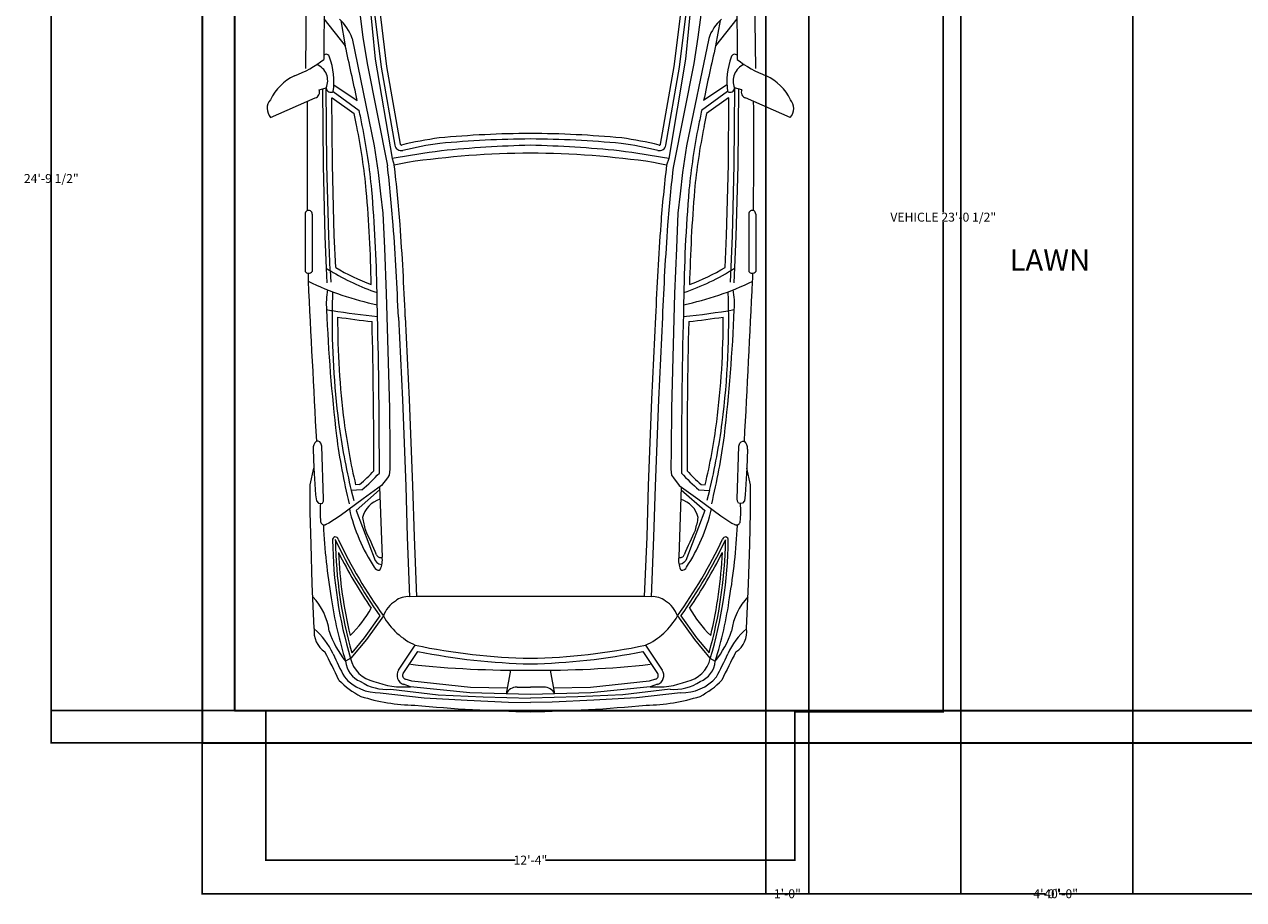
# Model space of a CAD drawing. Units: inches. Extents: x 594 to 1173, y 353 to 1285.
# Tile 1 of 6: x 594 to 934, y 355 to 600. Entities that reach past the tile are written whole.
import ezdxf

# ---------------------------------------------------------------- set-up
doc = ezdxf.new("R2010")
doc.units = ezdxf.units.IN
doc.header["$MEASUREMENT"] = 0
for name, color, linetype, lineweight in [('A-ANNO-DIMS', 2, 'Continuous', 18), ('A-AREA-IDEN', 7, 'Continuous', 25), ('C-PRKG-VEHI', 8, 'Continuous', 13), ('C-PROP', 7, 'Continuous', 35)]:
    doc.layers.add(name, color=color, linetype=linetype, lineweight=lineweight)
doc.styles.get("Standard").update_dxf_attribs({"font": 'arial.ttf'})
doc.dimstyles.get("Standard").update_dxf_attribs({"dimtxt": 2.5, "dimasz": 0.18, "dimexe": 0.18, "dimexo": 0.0625, "dimgap": 0.09, "dimtad": 0, "dimtih": 1, "dimtoh": 1, "dimzin": 0, "dimdsep": 46, "dimlunit": 3, "dimtxsty": 'Standard', "dimcen": 0.09, "dimadec": 0, "dimazin": 0, "dimtfac": 1, "dimtofl": 0, "dimtmove": 0, "dimatfit": 3, "dimfxl": 1, "dimtolj": 1, "dimtzin": 0, "dimarcsym": 0})

# ---------------------------------------------------------------- blocks, each defined once
blk = doc.blocks.new('A$C27D64469')
for p, q in [((-0.6398, -1.1535), (-0.5904, -1.5351)), ((-0.5908, -1.1535), (-0.5454, -1.6151)), ((0.618, -1.1535), (0.5726, -1.6151)), ((0.6669, -1.1535), (0.6175, -1.5351)), ((-0.563, -1.3311), (-0.5244, -1.6438)), ((-0.5431, -1.3287), (-0.5046, -1.6408)), ((0.5317, -1.6408), (0.5703, -1.3287)), ((0.5515, -1.6438), (0.5901, -1.3311)), ((-0.7946, -1.3764), (-0.7975, -1.6481)), ((-0.7302, -1.3933), (-0.7314, -1.6155)), ((0.7573, -1.3933), (0.7586, -1.6155)), ((0.8217, -1.3764), (0.8246, -1.6481)), ((-0.7306, -1.4695), (-0.6539, -1.5666)), ((-0.6702, -1.4746), (-0.6539, -1.5666)), ((0.7578, -1.4695), (0.681, -1.5666)), ((0.6973, -1.4746), (0.681, -1.5666)), ((-0.5904, -1.5351), (-0.5754, -1.6301)), ((0.6175, -1.5351), (0.6026, -1.6301)), ((-0.6294, -1.5396), (-0.5492, -1.9272)), ((0.6565, -1.5396), (0.5764, -1.9272)), ((-0.5454, -1.6151), (-0.4851, -1.9723)), ((0.5726, -1.6151), (0.5122, -1.9723)), ((-0.5754, -1.6301), (-0.5017, -1.9986)), ((-0.5244, -1.6438), (-0.475, -1.9247)), ((-0.5046, -1.6408), (-0.4553, -1.9213)), ((0.4824, -1.9213), (0.5317, -1.6408)), ((0.5021, -1.9247), (0.5515, -1.6438)), ((0.6026, -1.6301), (0.5289, -1.9986)), ((-0.6947, -1.7069), (-0.6109, -1.7637)), ((0.7218, -1.7069), (0.638, -1.7637)), ((-0.9228, -1.8245), (-0.7622, -1.7543)), ((-0.7483, -1.7248), (-0.7225, -1.7182)), ((-0.7364, -1.7217), (-0.7338, -1.998)), ((-0.7199, -1.9952), (-0.7225, -1.7182)), ((-0.6999, -1.9949), (-0.7021, -1.7537)), ((-0.7009, -1.7536), (-0.6216, -1.8108)), ((-0.6971, -1.7317), (-0.6035, -1.7992)), ((0.7242, -1.7317), (0.6307, -1.7992)), ((0.7281, -1.7536), (0.6487, -1.8108)), ((0.7271, -1.9949), (0.7293, -1.7537)), ((0.7496, -1.7182), (0.7471, -1.9952)), ((0.7755, -1.7248), (0.7496, -1.7182)), ((0.7635, -1.7217), (0.761, -1.998)), ((0.9499, -1.8245), (0.7893, -1.7543)), ((-0.5492, -1.9272), (-0.5351, -2.0233)), ((0.5764, -1.9272), (0.5623, -2.0233)), ((-0.4851, -1.9723), (-0.477, -1.9966)), ((0.5122, -1.9723), (0.5041, -1.9966)), ((-0.7338, -1.998), (-0.7273, -2.254)), ((-0.7134, -2.2512), (-0.7199, -1.9952)), ((-0.6934, -2.2505), (-0.6999, -1.9949)), ((0.7206, -2.2505), (0.7271, -1.9949)), ((0.7471, -1.9952), (0.7406, -2.2512)), ((0.761, -1.998), (0.7545, -2.254)), ((-0.5351, -2.0233), (-0.5266, -2.1005)), ((0.5623, -2.0233), (0.5538, -2.1005)), ((-0.5266, -2.1005), (-0.5182, -2.1702)), ((0.5538, -2.1005), (0.5453, -2.1702)), ((-0.7987, -2.1729), (-0.7987, -2.3802)), ((-0.7732, -2.1729), (-0.7732, -2.3802)), ((-0.5182, -2.1702), (-0.5125, -2.2965)), ((0.5453, -2.1702), (0.5397, -2.2965)), ((0.8003, -2.1729), (0.8003, -2.3802)), ((0.8259, -2.1729), (0.8259, -2.3802)), ((-0.7273, -2.254), (-0.7223, -2.368)), ((-0.7078, -2.3771), (-0.7134, -2.2512)), ((-0.6883, -2.3655), (-0.6934, -2.2505)), ((0.7155, -2.3655), (0.7206, -2.2505)), ((0.7406, -2.2512), (0.7332, -2.4181)), ((0.7545, -2.254), (0.7471, -2.4209)), ((-0.5125, -2.2965), (-0.5059, -2.4594)), ((0.5397, -2.2965), (0.5331, -2.4594)), ((-0.7223, -2.368), (-0.7199, -2.4209)), ((-0.7078, -2.3771), (-0.706, -2.4181)), ((-0.5059, -2.4594), (-0.4945, -2.8747)), ((0.5331, -2.4594), (0.5216, -2.8747)), ((-0.4622, -2.5454), (-0.4477, -2.8433)), ((-0.4375, -2.5434), (-0.423, -2.8413)), ((0.4646, -2.5434), (0.4501, -2.8413)), ((0.4894, -2.5454), (0.4748, -2.8433)), ((-0.4477, -2.8433), (-0.4357, -3.1539)), ((-0.423, -2.8413), (-0.4109, -3.152)), ((0.4501, -2.8413), (0.4381, -3.152)), ((0.4748, -2.8433), (0.4628, -3.1539)), ((-0.4945, -2.8747), (-0.4935, -3.0236)), ((0.5216, -2.8747), (0.5207, -3.0236)), ((-0.7694, -3.0205), (-0.7665, -3.0897)), ((-0.7516, -2.9924), (-0.758, -2.9914)), ((-0.7456, -2.9946), (-0.7516, -2.9924)), ((-0.7413, -2.9989), (-0.7456, -2.9946)), ((-0.738, -3.0096), (-0.7413, -2.9989)), ((-0.7319, -3.1994), (-0.738, -3.0096)), ((-0.4935, -3.0236), (-0.4926, -3.0933)), ((0.5207, -3.0236), (0.5197, -3.0933)), ((0.759, -3.1994), (0.7651, -3.0096)), ((0.7651, -3.0096), (0.7684, -2.9989)), ((0.7684, -2.9989), (0.7727, -2.9946)), ((0.7727, -2.9946), (0.7788, -2.9924)), ((0.7788, -2.9924), (0.7852, -2.9914)), ((0.7965, -3.0205), (0.7936, -3.0897)), ((-0.7802, -3.1498), (-0.7665, -3.0897)), ((-0.7665, -3.0897), (-0.761, -3.1849)), ((-0.4954, -3.115), (-0.502, -3.1244)), ((-0.4926, -3.0933), (-0.4954, -3.115)), ((0.5197, -3.0933), (0.5226, -3.115)), ((0.5226, -3.115), (0.5292, -3.1244)), ((0.7936, -3.0897), (0.7882, -3.1849)), ((0.8074, -3.1498), (0.7936, -3.0897)), ((-0.7802, -3.248), (-0.7802, -3.1498)), ((-0.6019, -3.1478), (-0.6165, -3.1489)), ((-0.5227, -3.1517), (-0.5896, -3.1998)), ((-0.5302, -3.1571), (-0.5208, -3.4098)), ((-0.502, -3.1244), (-0.5227, -3.1517)), ((-0.4357, -3.1539), (-0.4303, -3.3385)), ((-0.4109, -3.152), (-0.4055, -3.3366)), ((0.4381, -3.152), (0.4327, -3.3366)), ((0.4628, -3.1539), (0.4574, -3.3385)), ((0.5292, -3.1244), (0.5499, -3.1517)), ((0.5573, -3.1571), (0.548, -3.4098)), ((0.5499, -3.1517), (0.6167, -3.1998)), ((0.6291, -3.1478), (0.6437, -3.1489)), ((0.8074, -3.248), (0.8074, -3.1498)), ((-0.761, -3.1849), (-0.7577, -3.207)), ((-0.7577, -3.207), (-0.7506, -3.2153)), ((-0.7324, -3.2087), (-0.7319, -3.1994)), ((-0.5896, -3.1998), (-0.6725, -3.261)), ((-0.594, -3.1673), (-0.632, -3.1701)), ((-0.632, -3.1701), (-0.6229, -3.206)), ((-0.5298, -3.1676), (-0.615, -3.2421)), ((0.557, -3.1676), (0.6422, -3.2421)), ((0.6167, -3.1998), (0.6996, -3.261)), ((0.6212, -3.1673), (0.6592, -3.1701)), ((0.6592, -3.1701), (0.65, -3.206)), ((0.7595, -3.2087), (0.759, -3.1994)), ((0.7849, -3.207), (0.7778, -3.2153)), ((0.7882, -3.1849), (0.7849, -3.207)), ((-0.777, -3.3641), (-0.7802, -3.248)), ((-0.7506, -3.2153), (-0.743, -3.2171)), ((-0.743, -3.2171), (-0.7359, -3.2158)), ((-0.7359, -3.2158), (-0.7324, -3.2087)), ((-0.615, -3.2421), (-0.5463, -3.4221)), ((0.6422, -3.2421), (0.5734, -3.4221)), ((0.7631, -3.2158), (0.7595, -3.2087)), ((0.7702, -3.2171), (0.7631, -3.2158)), ((0.7778, -3.2153), (0.7702, -3.2171)), ((0.8042, -3.3641), (0.8074, -3.248)), ((-0.7224, -3.2921), (-0.7327, -3.2955)), ((-0.713, -3.2874), (-0.7233, -3.2925)), ((-0.6725, -3.261), (-0.713, -3.2874)), ((0.6996, -3.261), (0.7401, -3.2874)), ((0.7401, -3.2874), (0.7505, -3.2925)), ((0.7495, -3.2921), (0.7599, -3.2955)), ((-0.4303, -3.3385), (-0.4218, -3.5529)), ((-0.4055, -3.3366), (-0.3971, -3.5519)), ((0.4327, -3.3366), (0.4242, -3.5519)), ((0.4574, -3.3385), (0.449, -3.5529)), ((-0.7728, -3.5066), (-0.777, -3.3641)), ((0.8, -3.5066), (0.8042, -3.3641)), ((-0.5463, -3.4221), (-0.5397, -3.4296)), ((0.5734, -3.4221), (0.5668, -3.4296)), ((-0.5397, -3.4296), (-0.5331, -3.4343)), ((-0.5331, -3.4343), (-0.5217, -3.4366)), ((0.5602, -3.4343), (0.5488, -3.4366)), ((0.5668, -3.4296), (0.5602, -3.4343)), ((-0.7654, -3.667), (-0.7728, -3.5066)), ((0.7926, -3.667), (0.8, -3.5066)), ((-0.3971, -3.5519), (-0.4218, -3.5529)), ((0.0136, -3.5519), (-0.3971, -3.5519)), ((0.4242, -3.5519), (0.0136, -3.5519)), ((0.449, -3.5529), (0.4242, -3.5519)), ((-0.5287, -3.6221), (-0.5854, -3.701)), ((-0.5163, -3.6221), (-0.5774, -3.7071)), ((0.5435, -3.6221), (0.6046, -3.7071)), ((0.5559, -3.6221), (0.6126, -3.701)), ((-0.5774, -3.7071), (-0.6331, -3.7742)), ((-0.5854, -3.701), (-0.6302, -3.755)), ((-0.4616, -3.818), (-0.4014, -3.7275)), ((0.4285, -3.7275), (0.4887, -3.818)), ((0.6046, -3.7071), (0.6602, -3.7742)), ((0.6126, -3.701), (0.6574, -3.755)), ((-0.6331, -3.7742), (-0.6525, -3.7849)), ((-0.4449, -3.8291), (-0.3922, -3.7498)), ((0.4193, -3.7498), (0.4721, -3.8291)), ((0.6602, -3.7742), (0.6796, -3.7849)), ((-0.0581, -3.8176), (-0.0735, -3.9028)), ((0.0853, -3.8176), (0.1006, -3.9028)), ((-0.4142, -3.8575), (-0.4379, -3.8496)), ((-0.2029, -3.8795), (-0.4142, -3.8575)), ((0.4414, -3.8575), (0.2301, -3.8795)), ((0.465, -3.8496), (0.4414, -3.8575)), ((-0.5278, -3.8988), (-0.3693, -3.9174)), ((-0.4897, -3.8861), (-0.3195, -3.9066)), ((-0.4185, -3.8772), (-0.4442, -3.8686)), ((-0.2042, -3.8994), (-0.4185, -3.8772)), ((-0.3195, -3.9066), (-0.1571, -3.9135)), ((0.0136, -3.905), (-0.2042, -3.8994)), ((-0.0699, -3.8829), (-0.2029, -3.8795)), ((-0.0347, -3.8792), (0.0136, -3.8792)), ((0.0618, -3.8792), (0.0136, -3.8792)), ((0.2314, -3.8994), (0.0136, -3.905)), ((0.2301, -3.8795), (0.097, -3.8829)), ((0.3466, -3.9066), (0.1842, -3.9135)), ((0.4456, -3.8772), (0.2314, -3.8994)), ((0.5168, -3.8861), (0.3466, -3.9066)), ((0.5549, -3.8988), (0.3965, -3.9174)), ((0.4713, -3.8686), (0.4456, -3.8772)), ((-0.3693, -3.9174), (-0.2148, -3.9262)), ((-0.2148, -3.9262), (-0.0652, -3.933)), ((-0.1571, -3.9135), (0.0136, -3.9184)), ((-0.0652, -3.933), (0.0136, -3.934)), ((0.1842, -3.9135), (0.0136, -3.9184)), ((0.0923, -3.933), (0.0136, -3.934)), ((0.242, -3.9262), (0.0923, -3.933)), ((0.3965, -3.9174), (0.242, -3.9262))]:
    blk.add_line(p, q)
for centre, radius, start, end in [((-0.7826, -1.5905), 0.1615, 18.3646, 48.2784), ((0.8098, -1.5905), 0.1615, 131.7216, 161.6354), ((-10.825, -3.8887), 10.4328, 11.75206, 12.86028), ((10.8521, -3.8887), 10.4328, 167.13972, 168.24794), ((-0.9818, -1.2945), 0.4071, 290.8732, 307.9458), ((-0.7227, -1.6094), 0.0124, 11.3416, 134.5987), ((-0.9441, -1.6953), 0.2497, 351.6082, 20.7105), ((0.9712, -1.6953), 0.2497, 159.2895, 188.3918), ((0.7498, -1.6094), 0.0124, 45.4013, 168.6584), ((1.0089, -1.2945), 0.4071, 232.0542, 249.1268), ((-0.7801, -1.6924), 0.0631, 335.8522, 68.2516), ((0.8072, -1.6924), 0.0631, 111.7484, 204.1478), ((-0.7607, -1.8385), 0.1804, 114.9135, 154.5523), ((0.7879, -1.8385), 0.1804, 25.4477, 65.0865), ((-0.7685, -1.7333), 0.0219, 286.784, 22.9417), ((-0.7054, -1.7168), 0.0171, 184.6651, 299.1967), ((-0.7054, -1.7168), 0.0371, 275.0842, 276.9824), ((0.7326, -1.7168), 0.0171, 240.8033, 355.3349), ((0.7326, -1.7168), 0.0371, 263.0176, 264.9158), ((0.7957, -1.7333), 0.0219, 157.0583, 253.216), ((-0.8877, -1.7923), 0.0477, 138.9599, 222.5475), ((28.5723, -1.9291), 29.3639, 179.68363, 180.45247), ((-10.825, -3.8887), 10.4328, 11.24656, 11.5533), ((10.8521, -3.8887), 10.4328, 168.4467, 168.75344), ((-28.5452, -1.9291), 29.3639, 359.54753, 0.31637), ((0.9148, -1.7923), 0.0477, 317.4525, 41.0401), ((-10.825, -3.8887), 10.4128, 11.24635, 11.51036), ((10.8521, -3.8887), 10.4128, 168.48964, 168.75365), ((-2.7812, -2.2979), 2.2132, 5.4405, 11.4681), ((-2.7812, -2.2979), 2.2332, 5.4374, 11.4671), ((0.034, -5.6085), 3.7262, 90.3146, 95.3817), ((-0.0069, -5.6085), 3.7262, 84.6183, 89.6854), ((2.8083, -2.2979), 2.2332, 168.5329, 174.5626), ((2.8083, -2.2979), 2.2132, 168.5319, 174.5595), ((-0.4518, -1.9207), 0.0236, 189.9743, 283.4471), ((-0.4518, -1.9207), 0.00357, 189.9743, 283.4471), ((-0.1284, -3.2729), 1.3868, 97.7498, 103.4471), ((-0.1284, -3.2729), 1.3668, 97.7671, 103.4471), ((0.034, -5.6085), 3.7062, 90.3163, 95.3753), ((0.1214, -6.2334), 4.3098, 91.434, 95.7038), ((-0.0069, -5.6085), 3.7062, 84.6247, 89.6837), ((-0.0943, -6.2334), 4.3098, 84.2962, 88.566), ((0.1556, -3.2729), 1.3668, 76.5529, 82.2329), ((0.1556, -3.2729), 1.3868, 76.5529, 82.2502), ((0.4789, -1.9207), 0.0236, 256.5529, 350.0257), ((0.4789, -1.9207), 0.00357, 256.5529, 350.0257), ((2.8455, -23.0231), 21.3127, 98.50598, 98.99062), ((0.0355, -5.2091), 3.2558, 90.3851, 98.2136), ((-0.0083, -5.2091), 3.2558, 81.7864, 89.6149), ((-2.8184, -23.0231), 21.3127, 81.00938, 81.49402), ((-6.4408, -2.6841), 5.9785, 4.51893, 6.58421), ((-0.0958, -3.6836), 1.7295, 101.1311, 102.7329), ((-6.416, -2.6821), 5.9785, 4.51893, 6.58421), ((0.1229, -3.6836), 1.7295, 77.2671, 78.8689), ((6.4432, -2.6821), 5.9785, 173.41579, 175.48107), ((6.4679, -2.6841), 5.9785, 173.41579, 175.48107), ((-6.2705, -2.56), 5.7121, 1.3286, 4.7387), ((-6.2705, -2.56), 5.7321, 1.03863, 4.73991), ((6.2976, -2.56), 5.7321, 175.26009, 179.33379), ((6.2976, -2.56), 5.7121, 175.2613, 178.6714), ((-0.7859, -2.1729), 0.0128, 359.8097, 180.1903), ((0.8131, -2.1729), 0.0128, 359.8097, 180.1903), ((-11.1621, -2.9794), 10.7086, 2.32274, 4.10377), ((-11.1373, -2.9775), 10.7086, 2.32274, 4.10377), ((11.1645, -2.9775), 10.7086, 175.89623, 177.67726), ((11.1892, -2.9794), 10.7086, 175.89623, 177.67726), ((-0.2816, -1.6867), 0.8114, 237.1024, 238.3082), ((-0.2816, -1.6867), 0.7914, 239.0709, 249.4088), ((0.3087, -1.6867), 0.8114, 288.5207, 302.8976), ((0.3087, -1.6867), 0.7914, 290.5912, 300.9291), ((-0.7859, -2.3704), 0.0161, 217.6419, 322.3581), ((28.5723, -1.9291), 29.3639, 180.89229, 180.9487), ((145.5619, 4.7984), 146.5271, 182.82189, 183.047472), ((-0.3074, -1.4152), 1.1094, 244.3519, 257.9711), ((-0.2816, -1.6867), 0.8114, 238.3082, 251.4793), ((0.3345, -1.4152), 1.1094, 282.0289, 295.6481), ((-145.5348, 4.7984), 146.5271, 356.952528, 357.17811), ((0.8131, -2.3704), 0.0161, 217.6419, 322.3581), ((-28.5452, -1.9291), 29.3639, 359.0513, 359.10771), ((-0.4463, -2.4963), 0.2758, 169.4971, 184.519), ((2.1845, -2.5566), 2.8858, 177.9428, 179.2929), ((-6.2705, -2.56), 5.7321, 0.66621, 1.03863), ((-2.1573, -2.5566), 2.8858, 352.6735, 2.0572), ((0.4735, -2.4963), 0.2758, 355.481, 10.5029), ((-21.144, -3.0635), 20.6131, 1.44842, 1.58522), ((21.1711, -3.0635), 20.6131, 178.41478, 180.12035), ((-0.2547, 0.2402), 2.7971, 260.3968, 260.8181), ((5.4584, -2.2589), 6.1852, 182.40058, 186.62429), ((2.1845, -2.5566), 2.8858, 179.2929, 187.3265), ((-0.2547, 0.2402), 2.7971, 260.8181, 264.1988), ((-0.2547, 0.2402), 2.8171, 261.2916, 263.8402), ((2.1845, -2.5566), 2.8658, 179.7551, 187.3262), ((-21.144, -3.0635), 20.6131, 359.87965, 1.44842), ((0.2819, 0.2402), 2.7971, 275.8012, 279.6032), ((0.2819, 0.2402), 2.8171, 276.1598, 278.7084), ((-2.1573, -2.5566), 2.8658, 352.6738, 0.2449), ((-5.4313, -2.2589), 6.1852, 353.37571, 357.59942), ((-21.144, -3.0635), 20.5931, 359.90118, 1.39956), ((21.1711, -3.0635), 20.5931, 178.60044, 180.09882), ((1.5917, -2.6291), 2.2886, 187.4191, 193.6744), ((1.5917, -2.6291), 2.2686, 187.4195, 193.2465), ((-1.5646, -2.6291), 2.2686, 346.7535, 352.5805), ((-1.5646, -2.6291), 2.2886, 346.3256, 352.5809), ((1.584, -2.6769), 2.2886, 187.4191, 193.6744), ((-1.5568, -2.6769), 2.2886, 346.3256, 352.5809), ((-0.7323, -3.0182), 0.0371, 133.8458, 183.4773), ((0.7594, -3.0182), 0.0371, 356.5227, 46.1542), ((-0.9762, -2.7051), 0.5797, 310.2112, 317.1922), ((-0.9762, -2.7051), 0.5997, 309.5861, 317.9444), ((1.0033, -2.7051), 0.5997, 222.0556, 230.4139), ((1.0033, -2.7051), 0.5797, 222.8078, 229.7888), ((-0.5023, -3.2896), 0.0919, 106.6274, 166.1462), ((0.5294, -3.2896), 0.0919, 13.8538, 73.3726), ((-0.4258, -3.2462), 0.3189, 174.7532, 186.4501), ((-0.0025, -3.0882), 0.6536, 193.0984, 213.2489), ((0.0296, -3.0882), 0.6536, 326.7511, 346.9016), ((0.4529, -3.2462), 0.3189, 353.5499, 5.2468), ((-0.7293, -3.2805), 0.0135, 186.4501, 296.5725), ((1.5487, -3.1796), 2.2844, 182.9075, 189.515), ((-0.2573, -3.2127), 0.3386, 189.3185, 197.018), ((0.2844, -3.2127), 0.3386, 342.982, 350.6815), ((-1.5216, -3.1796), 2.2844, 350.485, 357.0925), ((0.7565, -3.2805), 0.0135, 243.4275, 353.5499), ((-0.6895, -3.3475), 0.0103, 9.7306, 189.7306), ((-6.7047, -6.1366), 6.7437, 23.9284, 24.763), ((6.7318, -6.1366), 6.7437, 155.237, 156.0716), ((0.7166, -3.3475), 0.0103, 350.2694, 170.2694), ((0.8768, -3.3275), 1.5766, 180.7904, 196.499), ((-0.6895, -3.3475), 0.000207, 234.3096, 189.7306), ((-0.6997, -3.3492), 0.0101, 0.7904, 9.7306), ((0.9825, -2.5519), 1.8518, 205.4494, 215.3046), ((0.8768, -3.3275), 1.5665, 180.7904, 195.8378), ((0.9825, -2.5519), 1.8417, 205.5332, 215.5287), ((-0.9554, -2.5519), 1.8417, 324.4713, 334.4668), ((-0.9554, -2.5519), 1.8518, 324.6954, 334.5506), ((-0.8496, -3.3275), 1.5665, 344.1622, 359.2096), ((-0.8496, -3.3275), 1.5766, 343.501, 359.2096), ((0.7166, -3.3475), 0.000207, 350.2694, 305.6904), ((0.7268, -3.3492), 0.0101, 170.2694, 179.2096), ((0.8768, -3.3275), 1.5564, 182.4426, 193.5531), ((0.9825, -2.5519), 1.8619, 206.8832, 214.0379), ((-0.5273, -3.3975), 0.0139, 196.0998, 297.49), ((-0.5991, -3.4208), 0.079, 335.0797, 7.9846), ((0.6263, -3.4208), 0.079, 172.0154, 204.9203), ((0.5544, -3.3975), 0.0139, 242.51, 343.9002), ((-0.9554, -2.5519), 1.8619, 325.9621, 333.1168), ((-0.8496, -3.3275), 1.5564, 346.4469, 357.5574), ((-0.5332, -3.4402), 0.0172, 201.6995, 279.6425), ((-0.5326, -3.4521), 0.00559, 294.9923, 338.6694), ((0.5598, -3.4521), 0.00559, 201.3306, 245.0077), ((0.5603, -3.4402), 0.0172, 260.3575, 338.3005), ((-0.931, -3.7054), 0.2213, 7.498, 43.5729), ((0.6722, -3.364), 1.3899, 187.9913, 197.6257), ((-0.4293, -3.6198), 0.0673, 83.5915, 130.4352), ((0.4565, -3.6198), 0.0673, 49.5648, 96.4085), ((-0.645, -3.364), 1.3899, 342.3743, 352.0087), ((0.9581, -3.7054), 0.2213, 136.4271, 172.502), ((-0.9014, -3.4088), 0.388, 313.0938, 331.4872), ((-0.421, -3.6549), 0.1008, 121.0416, 161.032), ((0.4482, -3.6549), 0.1008, 18.968, 58.9584), ((0.9285, -3.4088), 0.388, 208.5128, 226.9062), ((-0.3005, -3.502), 0.247, 209.0915, 245.8956), ((0.3276, -3.502), 0.247, 294.1044, 330.9085), ((-0.6785, -3.679), 0.0877, 172.132, 236.2396), ((-0.9429, -3.8711), 0.2695, 24.6265, 48.8595), ((-0.3962, -3.5747), 0.3315, 197.8909, 219.3552), ((0.4233, -3.5747), 0.3315, 320.6448, 342.1091), ((0.97, -3.8711), 0.2695, 131.1405, 155.3735), ((0.7057, -3.679), 0.0877, 303.7604, 7.868), ((0.0567, -1.5526), 2.2226, 258.1061, 268.8881), ((-0.0296, -1.5526), 2.2226, 271.1119, 281.8939), ((-3.375, -5.1387), 2.9889, 25.4724, 27.6425), ((0.5567, -3.1915), 1.3769, 204.3314, 208.2014), ((-0.528, -3.7506), 0.1097, 192.9436, 258.3207), ((0.0567, -1.5526), 2.2426, 258.453, 268.898), ((-0.0296, -1.5526), 2.2426, 271.102, 281.547), ((0.5551, -3.7506), 0.1097, 281.6793, 347.0564), ((-0.5295, -3.1915), 1.3769, 331.7986, 335.6686), ((3.4021, -5.1387), 2.9889, 152.3575, 154.5276), ((-0.566, -3.7782), 0.0867, 184.4324, 248.21), ((-0.4335, -3.8367), 0.0337, 146.3764, 251.5583), ((-0.0346, -0.3333), 3.4843, 263.6749, 270.7924), ((0.0618, -0.3333), 3.4843, 269.2076, 276.3251), ((0.4607, -3.8367), 0.0337, 288.4417, 33.6236), ((0.5932, -3.7782), 0.0867, 291.79, 355.5676), ((-0.4633, -3.6496), 0.2949, 223.6549, 242.8613), ((-0.5341, -3.738), 0.1609, 220.3568, 272.2613), ((-0.5047, -3.7168), 0.17, 236.6049, 275.0704), ((-0.4436, -3.5867), 0.2916, 248.5479, 274.9353), ((-0.4335, -3.8367), 0.0137, 146.3764, 251.5583), ((0.4707, -3.5867), 0.2916, 265.0647, 291.4521), ((0.4607, -3.8367), 0.0137, 288.4417, 33.6236), ((0.5318, -3.7168), 0.17, 264.9296, 303.3951), ((0.5613, -3.738), 0.1609, 267.7387, 319.6432), ((0.4904, -3.6496), 0.2949, 297.1387, 316.3451), ((-0.0379, -3.9176), 0.0386, 85.1824, 157.357), ((0.065, -3.9176), 0.0386, 22.643, 94.8176), ((-0.3932, -3.2709), 0.673, 252.2974, 269.1096), ((0.1171, 1.5736), 5.542, 264.6089, 268.93), ((-0.0899, 1.5736), 5.542, 271.07, 275.3911), ((0.4203, -3.2709), 0.673, 270.8904, 287.7026)]:
    blk.add_arc(centre, radius, start, end)
blk = doc.blocks.new('*D44')
at = {"layer": 'A-ANNO-DIMS', "color": 0, "lineweight": -2, "transparency": 16777216}
for p, q in [((808.99, 683.97), (850.58, 683.97)), ((850.4, 683.79), (850.4, 547.1)), ((850.4, 407.65), (850.4, 544.34)), ((808.99, 407.47), (850.58, 407.47))]:
    blk.add_line(p, q, dxfattribs=at)
at = {"layer": 'A-ANNO-DIMS', "color": 0, "transparency": 16777216}
for points in [[(850.37, 683.79), (850.43, 683.79), (850.4, 683.97)], [(850.37, 407.65), (850.43, 407.65), (850.4, 407.47)]]:
    blk.add_solid(points, dxfattribs=at)
at = {"layer": 'Defpoints', "color": 0, "transparency": 16777216}
for p in [(808.93, 683.97), (850.4, 683.97), (808.93, 407.47)]:
    blk.add_point(p, dxfattribs=at)
at = {"layer": 'A-ANNO-DIMS', "color": 0, "transparency": 16777216, "insert": (850.4, 545.72), "char_height": 2.5, "attachment_point": 5}
blk.add_mtext('\\A1;VEHICLE 23\'-0 1/2"', dxfattribs=at)
blk = doc.blocks.new('*D45')
at = {"layer": 'A-ANNO-DIMS', "color": 0, "lineweight": -2, "transparency": 16777216}
for p, q in [((661.13, 407.41), (661.13, 365.81)), ((808.93, 407.41), (808.93, 365.81)), ((661.31, 365.99), (730.76, 365.99)), ((808.75, 365.99), (739.29, 365.99))]:
    blk.add_line(p, q, dxfattribs=at)
at = {"layer": 'A-ANNO-DIMS', "color": 0, "transparency": 16777216}
for points in [[(661.31, 366.02), (661.31, 365.96), (661.13, 365.99)], [(808.75, 366.02), (808.75, 365.96), (808.93, 365.99)]]:
    blk.add_solid(points, dxfattribs=at)
at = {"layer": 'Defpoints', "color": 0, "transparency": 16777216}
for p in [(661.13, 407.47), (808.93, 407.47), (808.93, 365.99)]:
    blk.add_point(p, dxfattribs=at)
at = {"layer": 'A-ANNO-DIMS', "color": 0, "transparency": 16777216, "insert": (735.03, 365.99), "char_height": 2.5, "attachment_point": 5}
blk.add_mtext('\\A1;12\'-4"', dxfattribs=at)
blk = doc.blocks.new('*D46')
at = {"layer": 'A-ANNO-DIMS', "color": 0, "lineweight": -2, "transparency": 16777216}
for p, q in [((643.34, 398.72), (643.34, 356.4)), ((1123.34, 398.72), (1123.34, 356.4)), ((643.52, 356.58), (878.9, 356.58)), ((1123.16, 356.58), (887.77, 356.58))]:
    blk.add_line(p, q, dxfattribs=at)
at = {"layer": 'A-ANNO-DIMS', "color": 0, "transparency": 16777216}
for points in [[(643.52, 356.61), (643.52, 356.55), (643.34, 356.58)], [(1123.16, 356.61), (1123.16, 356.55), (1123.34, 356.58)]]:
    blk.add_solid(points, dxfattribs=at)
at = {"layer": 'Defpoints', "color": 0, "transparency": 16777216}
for p in [(643.34, 398.78), (1123.34, 398.78), (1123.34, 356.58)]:
    blk.add_point(p, dxfattribs=at)
at = {"layer": 'A-ANNO-DIMS', "color": 0, "transparency": 16777216, "insert": (883.34, 356.58), "char_height": 2.5, "attachment_point": 5}
blk.add_mtext('\\A1;40\'-0"', dxfattribs=at)
blk = doc.blocks.new('*D47')
at = {"layer": 'A-ANNO-DIMS', "color": 0, "lineweight": -2, "transparency": 16777216}
for p, q in [((643.27, 1238.78), (600.96, 1238.78)), ((601.14, 1238.6), (601.14, 820.15)), ((601.14, 398.96), (601.14, 817.42)), ((643.27, 398.78), (600.96, 398.78))]:
    blk.add_line(p, q, dxfattribs=at)
at = {"layer": 'A-ANNO-DIMS', "color": 0, "transparency": 16777216}
for points in [[(601.11, 1238.6), (601.17, 1238.6), (601.14, 1238.78)], [(601.11, 398.96), (601.17, 398.96), (601.14, 398.78)]]:
    blk.add_solid(points, dxfattribs=at)
at = {"layer": 'Defpoints', "color": 0, "transparency": 16777216}
for p in [(601.14, 1238.78), (643.34, 1238.78), (643.34, 398.78)]:
    blk.add_point(p, dxfattribs=at)
at = {"layer": 'A-ANNO-DIMS', "color": 0, "transparency": 16777216, "insert": (601.14, 818.78), "char_height": 2.5, "attachment_point": 5}
blk.add_mtext('\\A1;70\'-0"', dxfattribs=at)
blk = doc.blocks.new('*D56')
at = {"layer": 'A-ANNO-DIMS', "color": 0, "lineweight": -2, "transparency": 16777216}
for p, q in [((652.27, 705.28), (600.96, 705.28)), ((601.14, 705.1), (601.14, 557.92)), ((601.14, 407.96), (601.14, 555.15)), ((652.27, 407.78), (600.96, 407.78))]:
    blk.add_line(p, q, dxfattribs=at)
at = {"layer": 'A-ANNO-DIMS', "color": 0, "transparency": 16777216}
for points in [[(601.11, 705.1), (601.17, 705.1), (601.14, 705.28)], [(601.11, 407.96), (601.17, 407.96), (601.14, 407.78)]]:
    blk.add_solid(points, dxfattribs=at)
at = {"layer": 'Defpoints', "color": 0, "transparency": 16777216}
for p in [(601.14, 705.28), (652.34, 705.28), (652.34, 407.78)]:
    blk.add_point(p, dxfattribs=at)
at = {"layer": 'A-ANNO-DIMS', "color": 0, "transparency": 16777216, "insert": (601.14, 556.53), "char_height": 2.5, "attachment_point": 5}
blk.add_mtext('\\A1;24\'-9 1/2"', dxfattribs=at)
blk = doc.blocks.new('*D69')
at = {"layer": 'A-ANNO-DIMS', "color": 0, "lineweight": -2, "transparency": 16777216}
for p, q in [((855.34, 726.2), (855.34, 356.4)), ((903.34, 726.2), (903.34, 356.4)), ((855.52, 356.58), (875.87, 356.58)), ((903.16, 356.58), (882.8, 356.58))]:
    blk.add_line(p, q, dxfattribs=at)
at = {"layer": 'A-ANNO-DIMS', "color": 0, "transparency": 16777216}
for points in [[(855.52, 356.61), (855.52, 356.55), (855.34, 356.58)], [(903.16, 356.61), (903.16, 356.55), (903.34, 356.58)]]:
    blk.add_solid(points, dxfattribs=at)
at = {"layer": 'Defpoints', "color": 0, "transparency": 16777216}
for p in [(855.34, 726.26), (903.34, 726.26), (903.34, 356.58)]:
    blk.add_point(p, dxfattribs=at)
at = {"layer": 'A-ANNO-DIMS', "color": 0, "transparency": 16777216, "insert": (879.34, 356.58), "char_height": 2.5, "attachment_point": 5}
blk.add_mtext('\\A1;4\'-0"', dxfattribs=at)
blk = doc.blocks.new('*D73')
at = {"layer": 'A-ANNO-DIMS', "color": 0, "lineweight": -2, "transparency": 16777216}
for p, q in [((800.84, 870.22), (800.84, 356.4)), ((812.84, 870.22), (812.84, 356.4)), ((801.02, 356.58), (803.54, 356.58)), ((812.66, 356.58), (810.13, 356.58))]:
    blk.add_line(p, q, dxfattribs=at)
at = {"layer": 'A-ANNO-DIMS', "color": 0, "transparency": 16777216}
for points in [[(801.02, 356.61), (801.02, 356.55), (800.84, 356.58)], [(812.66, 356.61), (812.66, 356.55), (812.84, 356.58)]]:
    blk.add_solid(points, dxfattribs=at)
at = {"layer": 'Defpoints', "color": 0, "transparency": 16777216}
for p in [(800.84, 870.28), (812.84, 870.28), (812.84, 356.58)]:
    blk.add_point(p, dxfattribs=at)
at = {"layer": 'A-ANNO-DIMS', "color": 0, "transparency": 16777216, "insert": (806.84, 356.58), "char_height": 2.5, "attachment_point": 5}
blk.add_mtext('\\A1;1\'-0"', dxfattribs=at)

msp = doc.modelspace()

# ---------------------------------------------------------------- linework, layer by layer
at = {"layer": 'C-PROP'}
for p, q in [((643.337, 1238.783), (643.337, 398.783)), ((652.337, 1229.783), (652.337, 407.783)), ((652.337, 407.783), (1114.337, 407.783)), ((643.337, 398.783), (1123.337, 398.783))]:
    msp.add_line(p, q, dxfattribs=at)

# ---------------------------------------------------------------- block references
at = {"layer": 'C-PRKG-VEHI', "xscale": 77.53069963048091, "yscale": 77.53069963048091, "zscale": 77.53069963048091}
msp.add_blockref('A$C27D64469', (733.975, 715.065), dxfattribs=at)

# ---------------------------------------------------------------- texts
at = {"layer": 'A-AREA-IDEN'}
msp.add_text('LAWN', height=6, dxfattribs=at).set_placement((868.928, 530.726))

# ---------------------------------------------------------------- dimensions: what is measured, and where the dimension line sits
at = {"layer": 'A-ANNO-DIMS'}
for base, p1, p2, picture, middle in [((601.137, 1238.783), (643.337, 398.783), (643.337, 1238.783), '*D47', (601.137, 818.783)), ((601.137, 705.283), (652.337, 407.783), (652.337, 705.283), '*D56', (601.137, 556.533))]:
    dim = msp.add_linear_dim(base=base, p1=p1, p2=p2, angle=90, dimstyle='Standard', override={"dimdec": 1, "dimlfac": 1, "dimrnd": 0, "dimzin": 1, "dimdsep": 46, "dimlunit": 4, "dimfrac": 2}, dxfattribs=at)
    dim.commit()
    dim.dimension.update_dxf_attribs({"geometry": picture, "text_midpoint": middle})
for base, p1, p2, picture, middle in [((812.837, 356.583), (800.837, 870.283), (812.837, 870.283), '*D73', (806.837, 356.583)), ((903.337, 356.583), (855.337, 726.259), (903.337, 726.259), '*D69', (879.337, 356.583)), ((808.926, 365.992), (661.13, 407.468), (808.926, 407.468), '*D45', (735.028, 365.992)), ((1123.337, 356.583), (643.337, 398.783), (1123.337, 398.783), '*D46', (883.337, 356.583))]:
    dim = msp.add_linear_dim(base=base, p1=p1, p2=p2, dimstyle='Standard', override={"dimdec": 1, "dimlfac": 1, "dimrnd": 0, "dimzin": 1, "dimdsep": 46, "dimlunit": 4, "dimfrac": 2}, dxfattribs=at)
    dim.commit()
    dim.dimension.update_dxf_attribs({"geometry": picture, "text_midpoint": middle})
dim = msp.add_linear_dim(base=(850.401, 683.971), p1=(808.926, 407.468), p2=(808.926, 683.971), angle=90, text='VEHICLE <>', dimstyle='Standard', override={"dimdec": 1, "dimlfac": 1, "dimrnd": 0, "dimzin": 1, "dimdsep": 46, "dimlunit": 4, "dimfrac": 2}, dxfattribs=at)
dim.commit()
dim.dimension.update_dxf_attribs({"geometry": '*D44', "text_midpoint": (850.401, 545.719)})

doc.saveas('drawing.dxf')
